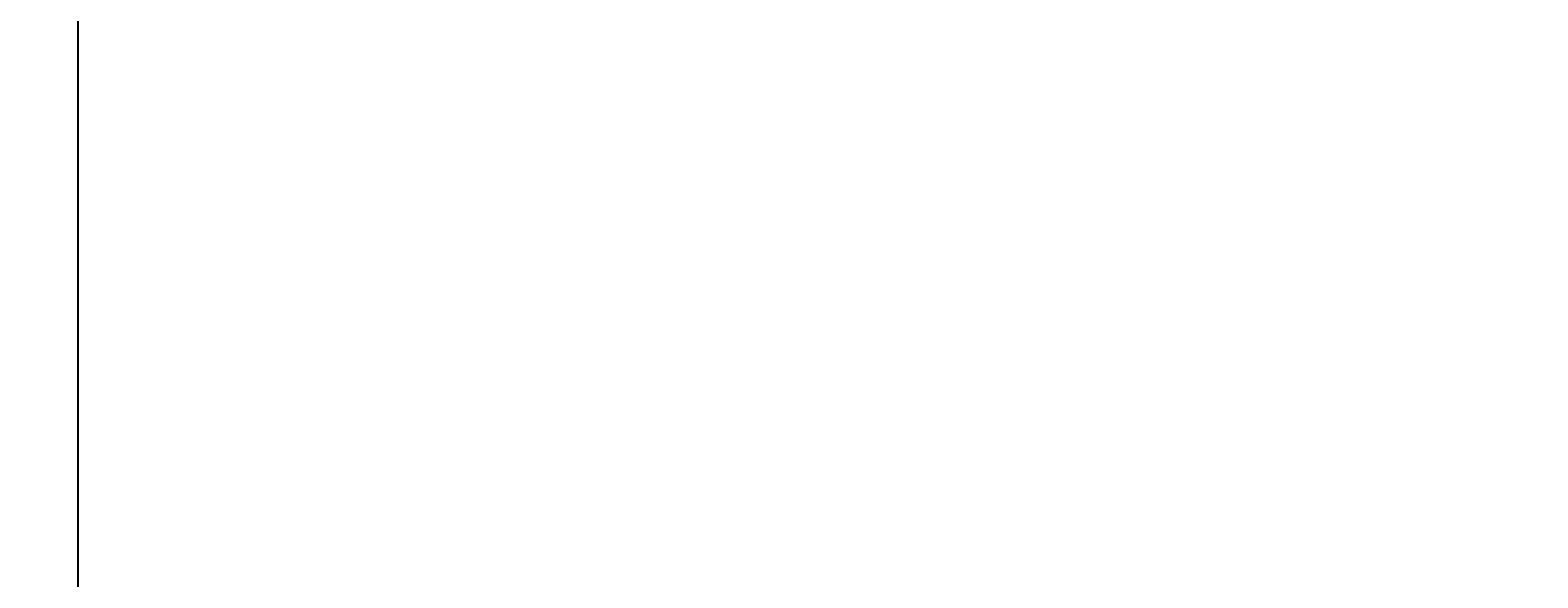
# Model space of a CAD drawing. Units: inches. Extents: x 35362 to 73946, y 43607 to 67532.
# Tile 105 of 134: x 50119 to 50761, y 49502 to 49735. Entities that reach past the tile are written whole.
import ezdxf

# ---------------------------------------------------------------- set-up
doc = ezdxf.new("R2010")
doc.units = ezdxf.units.IN
doc.header["$MEASUREMENT"] = 0
doc.layers.add('A-ANNO-DIMS', color=2, linetype='Continuous', lineweight=18)
doc.styles.get("Standard").update_dxf_attribs({"font": 'arial.ttf'})
doc.dimstyles.get("Standard").update_dxf_attribs({"dimtxt": 0.18, "dimasz": 0.18, "dimexe": 0.18, "dimexo": 0.0625, "dimgap": 0.09, "dimtad": 0, "dimtih": 1, "dimtoh": 1, "dimdec": 4, "dimzin": 0, "dimdsep": 46, "dimtxsty": 'Standard', "dimcen": 0.09, "dimadec": 0, "dimazin": 0, "dimtfac": 1, "dimtdec": 4, "dimtofl": 0, "dimtmove": 0, "dimatfit": 3, "dimfxl": 1, "dimtolj": 1, "dimtzin": 0, "dimarcsym": 0})

# ---------------------------------------------------------------- blocks, each defined once
blk = doc.blocks.new('*D11')
at = {"layer": 'A-ANNO-DIMS', "color": 0, "lineweight": -2, "transparency": 16777216}
for p, q in [((47978.66, 56028.77), (47978.66, 43606.68)), ((53109.76, 56028.77), (53109.76, 43606.68)), ((47978.84, 43606.86), (50543.87, 43606.86)), ((53109.58, 43606.86), (50544.55, 43606.86))]:
    blk.add_line(p, q, dxfattribs=at)
at = {"layer": 'A-ANNO-DIMS', "color": 0, "transparency": 16777216}
for points in [[(47978.84, 43606.89), (47978.84, 43606.83), (47978.66, 43606.86)], [(53109.58, 43606.89), (53109.58, 43606.83), (53109.76, 43606.86)]]:
    blk.add_solid(points, dxfattribs=at)
at = {"layer": 'Defpoints', "color": 0, "transparency": 16777216}
for p in [(47978.66, 56028.84), (53109.76, 56028.84), (53109.76, 43606.86)]:
    blk.add_point(p, dxfattribs=at)
at = {"layer": 'A-ANNO-DIMS', "color": 0, "transparency": 16777216, "insert": (50544.21, 43606.86), "char_height": 0.18, "attachment_point": 5}
blk.add_mtext('\\A1;5131', dxfattribs=at)
blk = doc.blocks.new('*D13')
at = {"layer": 'A-ANNO-DIMS', "color": 0, "lineweight": -2, "transparency": 16777216}
for p, q in [((48373.49, 51694.02), (48373.49, 43606.68)), ((51029.04, 51694.02), (51029.04, 43606.68)), ((48373.67, 43606.86), (49700.8, 43606.86)), ((51028.86, 43606.86), (49701.73, 43606.86))]:
    blk.add_line(p, q, dxfattribs=at)
at = {"layer": 'A-ANNO-DIMS', "color": 0, "transparency": 16777216}
for points in [[(48373.67, 43606.89), (48373.67, 43606.83), (48373.49, 43606.86)], [(51028.86, 43606.89), (51028.86, 43606.83), (51029.04, 43606.86)]]:
    blk.add_solid(points, dxfattribs=at)
at = {"layer": 'Defpoints', "color": 0, "transparency": 16777216}
for p in [(48373.49, 51694.09), (51029.04, 51694.09), (51029.04, 43606.86)]:
    blk.add_point(p, dxfattribs=at)
at = {"layer": 'A-ANNO-DIMS', "color": 0, "transparency": 16777216, "insert": (49701.27, 43606.86), "char_height": 0.18, "attachment_point": 5}
blk.add_mtext('\\A1;2655.6', dxfattribs=at)
blk = doc.blocks.new('*D17')
at = {"layer": 'A-ANNO-DIMS', "color": 0, "lineweight": -2, "transparency": 16777216}
for p, q in [((49923.31, 61293.22), (49923.31, 43606.68)), ((51913.93, 61293.22), (51913.93, 43606.68)), ((49923.49, 43606.86), (50918.16, 43606.86)), ((51913.75, 43606.86), (50919.07, 43606.86))]:
    blk.add_line(p, q, dxfattribs=at)
at = {"layer": 'A-ANNO-DIMS', "color": 0, "transparency": 16777216}
for points in [[(49923.49, 43606.89), (49923.49, 43606.83), (49923.31, 43606.86)], [(51913.75, 43606.89), (51913.75, 43606.83), (51913.93, 43606.86)]]:
    blk.add_solid(points, dxfattribs=at)
at = {"layer": 'Defpoints', "color": 0, "transparency": 16777216}
for p in [(49923.31, 61293.29), (51913.93, 61293.29), (51913.93, 43606.86)]:
    blk.add_point(p, dxfattribs=at)
at = {"layer": 'A-ANNO-DIMS', "color": 0, "transparency": 16777216, "insert": (50918.62, 43606.86), "char_height": 0.18, "attachment_point": 5}
blk.add_mtext('\\A1;1990.6', dxfattribs=at)
blk = doc.blocks.new('*D40')
at = {"layer": 'A-ANNO-DIMS', "color": 0, "lineweight": -2, "transparency": 16777216}
for p, q in [((56873.54, 53351.53), (35361.77, 53351.53)), ((35361.95, 53351.35), (35361.95, 51333.28)), ((35361.95, 49314.85), (35361.95, 51332.92)), ((51806.45, 49314.67), (35361.77, 49314.67))]:
    blk.add_line(p, q, dxfattribs=at)
at = {"layer": 'A-ANNO-DIMS', "color": 0, "transparency": 16777216}
for points in [[(35361.92, 53351.35), (35361.98, 53351.35), (35361.95, 53351.53)], [(35361.92, 49314.85), (35361.98, 49314.85), (35361.95, 49314.67)]]:
    blk.add_solid(points, dxfattribs=at)
at = {"layer": 'Defpoints', "color": 0, "transparency": 16777216}
for p in [(35361.95, 53351.53), (56873.6, 53351.53), (51806.52, 49314.67)]:
    blk.add_point(p, dxfattribs=at)
at = {"layer": 'A-ANNO-DIMS', "color": 0, "transparency": 16777216, "insert": (35361.95, 51333.1), "char_height": 0.18, "attachment_point": 5}
blk.add_mtext('\\A1;4036.9', dxfattribs=at)
blk = doc.blocks.new('*D67')
at = {"layer": 'A-ANNO-DIMS', "color": 0, "lineweight": -2, "transparency": 16777216}
for p, q in [((56873.54, 53351.53), (35361.77, 53351.53)), ((35361.95, 53351.35), (35361.95, 49400.89)), ((35361.95, 45450.07), (35361.95, 49400.53)), ((53793.58, 45449.89), (35361.77, 45449.89))]:
    blk.add_line(p, q, dxfattribs=at)
at = {"layer": 'A-ANNO-DIMS', "color": 0, "transparency": 16777216}
for points in [[(35361.92, 53351.35), (35361.98, 53351.35), (35361.95, 53351.53)], [(35361.92, 45450.07), (35361.98, 45450.07), (35361.95, 45449.89)]]:
    blk.add_solid(points, dxfattribs=at)
at = {"layer": 'Defpoints', "color": 0, "transparency": 16777216}
for p in [(35361.95, 53351.53), (56873.6, 53351.53), (53793.64, 45449.89)]:
    blk.add_point(p, dxfattribs=at)
at = {"layer": 'A-ANNO-DIMS', "color": 0, "transparency": 16777216, "insert": (35361.95, 49400.71), "char_height": 0.18, "attachment_point": 5}
blk.add_mtext('\\A1;7901.6', dxfattribs=at)
blk = doc.blocks.new('*D107')
at = {"layer": 'A-ANNO-DIMS', "color": 0, "lineweight": -2, "transparency": 16777216}
for p, q in [((50139.56, 59850.01), (50139.56, 43606.68)), ((51320.81, 59850.01), (51320.81, 43606.68)), ((50139.74, 43606.86), (50729.73, 43606.86)), ((51320.63, 43606.86), (50730.64, 43606.86))]:
    blk.add_line(p, q, dxfattribs=at)
at = {"layer": 'A-ANNO-DIMS', "color": 0, "transparency": 16777216}
for points in [[(50139.74, 43606.89), (50139.74, 43606.83), (50139.56, 43606.86)], [(51320.63, 43606.89), (51320.63, 43606.83), (51320.81, 43606.86)]]:
    blk.add_solid(points, dxfattribs=at)
at = {"layer": 'Defpoints', "color": 0, "transparency": 16777216}
for p in [(50139.56, 59850.08), (51320.81, 59850.08), (51320.81, 43606.86)]:
    blk.add_point(p, dxfattribs=at)
at = {"layer": 'A-ANNO-DIMS', "color": 0, "transparency": 16777216, "insert": (50730.19, 43606.86), "char_height": 0.18, "attachment_point": 5}
blk.add_mtext('\\A1;1181.3', dxfattribs=at)

msp = doc.modelspace()

# ---------------------------------------------------------------- dimensions: what is measured, and where the dimension line sits
at = {"layer": 'A-ANNO-DIMS'}
for base, p1, p2, override, picture, middle in [((51913.931, 43606.859), (49923.307, 61293.286), (51913.931, 61293.286), {"dimdec": 1, "dimlfac": 1, "dimrnd": 0, "dimzin": 0, "dimdsep": 46, "dimlunit": 2}, '*D17', (50918.619, 43606.859)), ((51320.8133, 43606.859), (50139.5627, 59850.0769), (51320.8133, 59850.0769), {"dimdec": 1, "dimlfac": 1, "dimrnd": 0, "dimzin": 0, "dimdsep": 46, "dimlunit": 2}, '*D107', (50730.188, 43606.859)), ((53109.76, 43606.859), (47978.665, 56028.836), (53109.76, 56028.836), {"dimdec": 0, "dimlfac": 1, "dimrnd": 0, "dimzin": 0, "dimdsep": 46, "dimlunit": 2}, '*D11', (50544.212, 43606.859)), ((51029.043, 43606.859), (48373.492, 51694.087), (51029.043, 51694.087), {"dimdec": 1, "dimlfac": 1, "dimrnd": 0, "dimzin": 0, "dimdsep": 46, "dimlunit": 2}, '*D13', (49701.267, 43606.859))]:
    dim = msp.add_linear_dim(base=base, p1=p1, p2=p2, dimstyle='Standard', override=override, dxfattribs=at)
    dim.commit()
    dim.dimension.update_dxf_attribs({"geometry": picture, "text_midpoint": middle})
for p1, picture, middle in [((51806.517, 49314.669), '*D40', (35361.949, 51333.099)), ((53793.638, 45449.894), '*D67', (35361.949, 49400.712))]:
    dim = msp.add_linear_dim(base=(35361.949, 53351.529), p1=p1, p2=(56873.602, 53351.529), angle=90, dimstyle='Standard', override={"dimdec": 1, "dimlfac": 1, "dimrnd": 0, "dimzin": 0, "dimdsep": 46, "dimlunit": 2}, dxfattribs=at)
    dim.commit()
    dim.dimension.update_dxf_attribs({"geometry": picture, "text_midpoint": middle})

doc.saveas('drawing.dxf')
